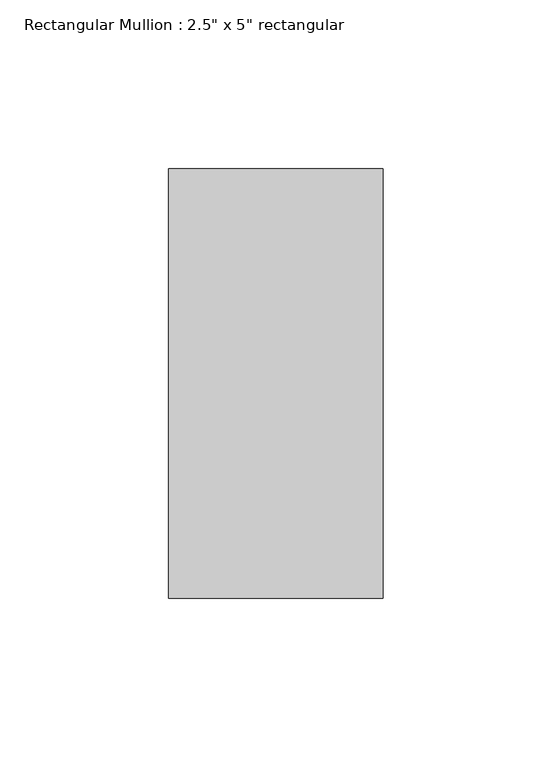
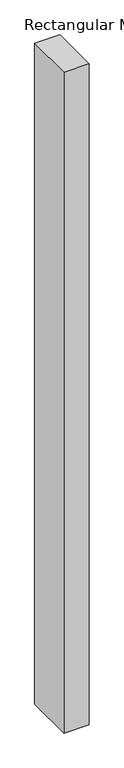
"""IFC4 building model written with IfcOpenShell, lengths in millimetres: member geometry."""

from ifc_helpers import new_model, si_unit, frame, origin, place, context, project, spatial, polyline, outline, extrude, source, transform, mapped, element, save


def member_2fbbe8c6(model_context):
    return source(origin(), model_context, "Body", "SweptSolid", [
        extrude(outline(polyline([(31.75, 63.5), (31.75, -63.5), (-31.75, -63.5), (-31.75, 63.5), (31.75, 63.5)])), frame((0.0, 0.0, -1755.4879691), z_axis=(0.0, 0.0, 1.0), x_axis=(1.0, 0.0, 0.0)), (0.0, 0.0, 1.0), 1755.4879691),
    ])


if __name__ == "__main__":
    model = new_model("IFC4")
    model_context = context("Model", 3, world=origin())
    ifc_project = project(units=[si_unit("LENGTHUNIT", "METRE", prefix="MILLI")], contexts=[model_context])
    site = spatial("IfcSite", under=ifc_project)
    building = spatial("IfcBuilding", under=site)
    placement = place(None, origin())
    member_shape = member_2fbbe8c6(model_context)
    element("IfcMember", 1, ObjectType="Rectangular Mullion : 2.5\" x 5\" rectangular", at=placement, inside=building, context=model_context, shape_type="MappedRepresentation", body=[
        mapped(member_shape, transform((0.0, 0.0, 0.0), x_axis=(1.0, 0.0, 0.0), y_axis=(0.0, 1.0, 0.0), z_axis=(0.0, 0.0, 1.0))),
    ])
    save(model, "model.ifc")

# Revit data of these elements
# Type "Rectangular Mullion : 2.5\" x 5\" rectangular"
#   built-in parameter 1007304 = 0.416667 (stored number, unit not read)
#   built-in parameter 1007301 = 0.104167 (stored number, unit not read)
#   built-in parameter 1007300 = 0.104167 (stored number, unit not read)
# Element 1 (IfcMember, "Rectangular Mullion : 2.5\" x 5\" rectangular")
#   Materials on its faces: "Aluminum"
# Materials
#   "Aluminum": class "Metal", colour RGB 247 247 247, transparency 0, Description = "Aluminum 6061", Cost = 0
